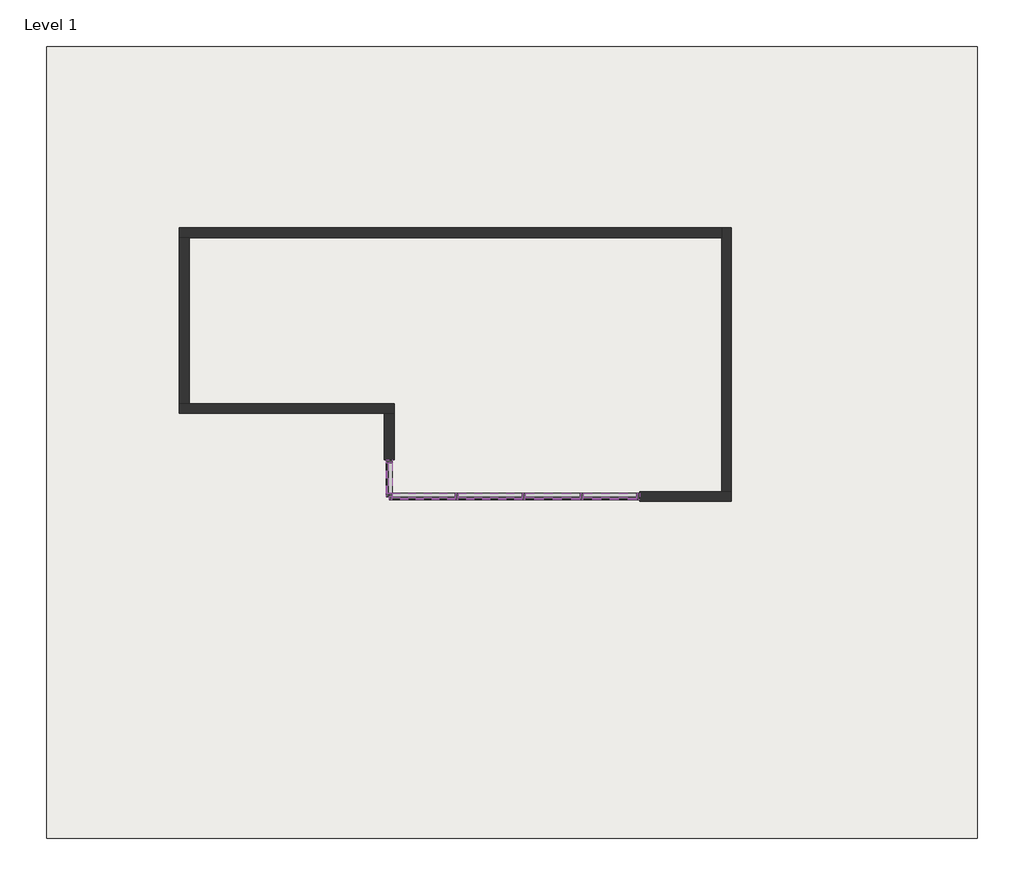
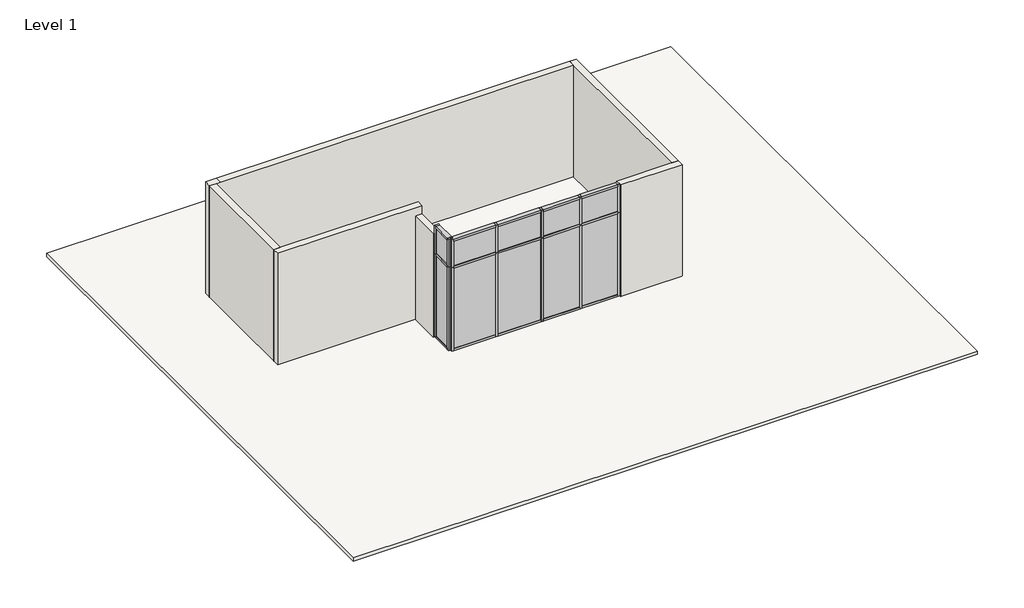
# One storey: 29 members, 10 plates, 6 walls, 1 slab.
"""IFC4 building model written with IfcOpenShell, lengths in millimetres."""

from ifc_helpers import new_model, si_unit, frame, origin, origin_with_axes, place, context, project, spatial, polyline, outline, extrude, faceted_brep, transform, mapped, element, save
from components import member_afc9459e, member_f32bdbca, member_44103a32, member_65750824, member_73c23c35, member_5e365d0c, member_923d5781, member_a78380a5, member_12300432, member_410c6227, member_d6aa3d2f, member_6609bf83, member_48e25eb9, member_c84aaad6, system_panel_glazed_120799d7, system_panel_glazed_8e2f599f, system_panel_glazed_26227597, system_panel_glazed_1d091053, system_panel_glazed_c9ee7fb0, system_panel_glazed_e21b380e, system_panel_glazed_be7f0fdb, system_panel_glazed_03477ef2, system_panel_glazed_aebd10dd, system_panel_glazed_a205a7ab

model = new_model("IFC4")

# Units and contexts
model_context = context("Model", 3, world=origin())
ifc_project = project(units=[si_unit("LENGTHUNIT", "METRE", prefix="MILLI")], contexts=[model_context])

# Site, building, storey
site = spatial("IfcSite", under=ifc_project)
building = spatial("IfcBuilding", under=site)
storey = spatial("IfcBuildingStorey", under=building, Name="Level 1", Elevation=0.0)

# Members
placement = place(None, origin())
member_shape = member_afc9459e(model_context)
element("IfcMember", 1, ObjectType="Rectangular Mullion : 2.5\" x 5\" rectangular", at=placement, inside=storey, context=model_context, shape_type="MappedRepresentation", body=[
    mapped(member_shape, transform((-8475.461895, 635.561619, 2743.2), x_axis=(0.0, 0.0, 1.0), y_axis=(0.0, 1.0, 0.0), z_axis=(-1.0, 0.0, 0.0))),
])
member_2_shape = member_f32bdbca(model_context)
element("IfcMember", 2, ObjectType="Rectangular Mullion : 2.5\" x 5\" rectangular", at=placement, inside=storey, context=model_context, shape_type="MappedRepresentation", body=[
    mapped(member_2_shape, transform((-8475.461895, 635.561619, 3657.6), x_axis=(0.0, 0.0, 1.0), y_axis=(0.0, 1.0, 0.0), z_axis=(-1.0, 0.0, 0.0))),
])
member_3_shape = member_44103a32(model_context)
element("IfcMember", 3, ObjectType="Rectangular Mullion : 2.5\" x 5\" rectangular", at=placement, inside=storey, context=model_context, shape_type="MappedRepresentation", body=[
    mapped(member_3_shape, transform((-9840.711895, 635.561619, 2743.2), x_axis=(0.0, 0.0, 1.0), y_axis=(0.0, 1.0, 0.0), z_axis=(-1.0, 0.0, 0.0))),
])
member_4_shape = member_65750824(model_context)
element("IfcMember", 4, ObjectType="Rectangular Mullion : 2.5\" x 5\" rectangular", at=placement, inside=storey, context=model_context, shape_type="MappedRepresentation", body=[
    mapped(member_4_shape, transform((-9840.711895, 635.561619, 3657.6), x_axis=(0.0, 0.0, 1.0), y_axis=(0.0, 1.0, 0.0), z_axis=(-1.0, 0.0, 0.0))),
])
member_5_shape = member_73c23c35(model_context)
element("IfcMember", 5, ObjectType="Rectangular Mullion : 2.5\" x 5\" rectangular", at=placement, inside=storey, context=model_context, shape_type="MappedRepresentation", body=[
    mapped(member_5_shape, transform((-9904.211895, 635.561619, 2743.2), x_axis=(-1.0, 0.0, 0.0), y_axis=(0.0, 1.0, 0.0), z_axis=(0.0, 0.0, -1.0))),
])
element("IfcMember", 6, ObjectType="Rectangular Mullion : 2.5\" x 5\" rectangular", at=placement, inside=storey, context=model_context, shape_type="MappedRepresentation", body=[
    mapped(member_5_shape, transform((-9904.211895, 1397.561619, 2743.2), x_axis=(0.0, 1.0, 0.0), y_axis=(1.0, 0.0, 0.0), z_axis=(0.0, 0.0, -1.0))),
])
member_6_shape = member_5e365d0c(model_context)
element("IfcMember", 7, ObjectType="Rectangular Mullion : 2.5\" x 5\" rectangular", at=placement, inside=storey, context=model_context, shape_type="MappedRepresentation", body=[
    mapped(member_6_shape, transform((-9904.211895, 1334.061619, 3657.6), x_axis=(0.0, 0.0, 1.0), y_axis=(1.0, 0.0, 0.0), z_axis=(0.0, 1.0, 0.0))),
])
element("IfcMember", 8, ObjectType="Rectangular Mullion : 2.5\" x 5\" rectangular", at=placement, inside=storey, context=model_context, shape_type="MappedRepresentation", body=[
    mapped(member_5_shape, transform((-9904.211895, 635.561619, 3657.6), x_axis=(0.0, -1.0, 0.0), y_axis=(1.0, 0.0, 0.0), z_axis=(0.0, 0.0, 1.0))),
])
element("IfcMember", 9, ObjectType="Rectangular Mullion : 2.5\" x 5\" rectangular", at=placement, inside=storey, context=model_context, shape_type="MappedRepresentation", body=[
    mapped(member_5_shape, transform((-4698.461546, 635.561619, 3657.6), x_axis=(1.0, 0.0, 0.0), y_axis=(0.0, 1.0, 0.0), z_axis=(0.0, 0.0, 1.0))),
])
member_7_shape = member_923d5781(model_context)
element("IfcMember", 10, ObjectType="Rectangular Mullion : 2.5\" x 5\" rectangular", at=placement, inside=storey, context=model_context, shape_type="MappedRepresentation", body=[
    mapped(member_7_shape, transform((-8507.211895, 635.561619, 0.0), x_axis=(-1.0, 0.0, 0.0), y_axis=(0.0, 1.0, 0.0), z_axis=(0.0, 0.0, -1.0))),
])
element("IfcMember", 11, ObjectType="Rectangular Mullion : 2.5\" x 5\" rectangular", at=placement, inside=storey, context=model_context, shape_type="MappedRepresentation", body=[
    mapped(member_7_shape, transform((-7110.211895, 635.561619, 0.0), x_axis=(-1.0, 0.0, 0.0), y_axis=(0.0, 1.0, 0.0), z_axis=(0.0, 0.0, -1.0))),
])
element("IfcMember", 12, ObjectType="Rectangular Mullion : 2.5\" x 5\" rectangular", at=placement, inside=storey, context=model_context, shape_type="MappedRepresentation", body=[
    mapped(member_7_shape, transform((-5904.3367205, 635.561619, 0.0), x_axis=(-1.0, 0.0, 0.0), y_axis=(0.0, 1.0, 0.0), z_axis=(0.0, 0.0, -1.0))),
])
element("IfcMember", 13, ObjectType="Rectangular Mullion : 2.5\" x 5\" rectangular", at=placement, inside=storey, context=model_context, shape_type="MappedRepresentation", body=[
    mapped(member_4_shape, transform((-8538.961895, 635.561619, 0.0), x_axis=(0.0, 0.0, -1.0), y_axis=(0.0, 1.0, 0.0), z_axis=(1.0, 0.0, 0.0))),
])
element("IfcMember", 14, ObjectType="Rectangular Mullion : 2.5\" x 5\" rectangular", at=placement, inside=storey, context=model_context, shape_type="MappedRepresentation", body=[
    mapped(member_2_shape, transform((-7141.961895, 635.561619, 0.0), x_axis=(0.0, 0.0, -1.0), y_axis=(0.0, 1.0, 0.0), z_axis=(1.0, 0.0, 0.0))),
])
member_8_shape = member_a78380a5(model_context)
element("IfcMember", 15, ObjectType="Rectangular Mullion : 2.5\" x 5\" rectangular", at=placement, inside=storey, context=model_context, shape_type="MappedRepresentation", body=[
    mapped(member_8_shape, transform((-9904.211895, 635.561619, 0.0), x_axis=(-1.0, 0.0, 0.0), y_axis=(0.0, 1.0, 0.0), z_axis=(0.0, 0.0, -1.0))),
])
element("IfcMember", 16, ObjectType="Rectangular Mullion : 2.5\" x 5\" rectangular", at=placement, inside=storey, context=model_context, shape_type="MappedRepresentation", body=[
    mapped(member_8_shape, transform((-9904.211895, 1397.561619, 0.0), x_axis=(0.0, 1.0, 0.0), y_axis=(1.0, 0.0, 0.0), z_axis=(0.0, 0.0, -1.0))),
])
element("IfcMember", 17, ObjectType="Rectangular Mullion : 2.5\" x 5\" rectangular", at=placement, inside=storey, context=model_context, shape_type="MappedRepresentation", body=[
    mapped(member_8_shape, transform((-4698.461546, 635.561619, 2743.2), x_axis=(1.0, 0.0, 0.0), y_axis=(0.0, 1.0, 0.0), z_axis=(0.0, 0.0, 1.0))),
])
element("IfcMember", 18, ObjectType="Rectangular Mullion : 2.5\" x 5\" rectangular", at=placement, inside=storey, context=model_context, shape_type="MappedRepresentation", body=[
    mapped(member_8_shape, transform((-9904.211895, 635.561619, 2743.2), x_axis=(0.0, -1.0, 0.0), y_axis=(1.0, 0.0, 0.0), z_axis=(0.0, 0.0, 1.0))),
])
element("IfcMember", 19, ObjectType="Rectangular Mullion : 2.5\" x 5\" rectangular", at=placement, inside=storey, context=model_context, shape_type="MappedRepresentation", body=[
    mapped(member_6_shape, transform((-9904.211895, 699.061619, 0.0), x_axis=(0.0, 0.0, -1.0), y_axis=(1.0, 0.0, 0.0), z_axis=(0.0, -1.0, 0.0))),
])
member_9_shape = member_12300432(model_context)
element("IfcMember", 20, ObjectType="Rectangular Mullion : 2.5\" x 5\" rectangular", at=placement, inside=storey, context=model_context, shape_type="MappedRepresentation", body=[
    mapped(member_9_shape, transform((-9904.211895, 1334.061619, 2743.2), x_axis=(0.0, 0.0, 1.0), y_axis=(1.0, 0.0, 0.0), z_axis=(0.0, 1.0, 0.0))),
])
member_10_shape = member_410c6227(model_context)
element("IfcMember", 21, ObjectType="Rectangular Mullion : 2.5\" x 5\" rectangular", at=placement, inside=storey, context=model_context, shape_type="MappedRepresentation", body=[
    mapped(member_10_shape, transform((-8507.211895, 635.561619, 2743.2), x_axis=(-1.0, 0.0, 0.0), y_axis=(0.0, 1.0, 0.0), z_axis=(0.0, 0.0, -1.0))),
])
element("IfcMember", 22, ObjectType="Rectangular Mullion : 2.5\" x 5\" rectangular", at=placement, inside=storey, context=model_context, shape_type="MappedRepresentation", body=[
    mapped(member_10_shape, transform((-7110.211895, 635.561619, 2743.2), x_axis=(-1.0, 0.0, 0.0), y_axis=(0.0, 1.0, 0.0), z_axis=(0.0, 0.0, -1.0))),
])
element("IfcMember", 23, ObjectType="Rectangular Mullion : 2.5\" x 5\" rectangular", at=placement, inside=storey, context=model_context, shape_type="MappedRepresentation", body=[
    mapped(member_10_shape, transform((-5904.3367205, 635.561619, 2743.2), x_axis=(-1.0, 0.0, 0.0), y_axis=(0.0, 1.0, 0.0), z_axis=(0.0, 0.0, -1.0))),
])
member_11_shape = member_d6aa3d2f(model_context)
element("IfcMember", 24, ObjectType="Rectangular Mullion : 2.5\" x 5\" rectangular", at=placement, inside=storey, context=model_context, shape_type="MappedRepresentation", body=[
    mapped(member_11_shape, transform((-5872.5867205, 635.561619, 2743.2), x_axis=(0.0, 0.0, 1.0), y_axis=(0.0, 1.0, 0.0), z_axis=(-1.0, 0.0, 0.0))),
])
member_12_shape = member_6609bf83(model_context)
element("IfcMember", 25, ObjectType="Rectangular Mullion : 2.5\" x 5\" rectangular", at=placement, inside=storey, context=model_context, shape_type="MappedRepresentation", body=[
    mapped(member_12_shape, transform((-7078.461895, 635.561619, 3657.6), x_axis=(0.0, 0.0, 1.0), y_axis=(0.0, 1.0, 0.0), z_axis=(-1.0, 0.0, 0.0))),
])
member_13_shape = member_48e25eb9(model_context)
element("IfcMember", 26, ObjectType="Rectangular Mullion : 2.5\" x 5\" rectangular", at=placement, inside=storey, context=model_context, shape_type="MappedRepresentation", body=[
    mapped(member_13_shape, transform((-4761.961546, 635.561619, 0.0), x_axis=(0.0, 0.0, -1.0), y_axis=(0.0, 1.0, 0.0), z_axis=(1.0, 0.0, 0.0))),
])
member_14_shape = member_c84aaad6(model_context)
element("IfcMember", 27, ObjectType="Rectangular Mullion : 2.5\" x 5\" rectangular", at=placement, inside=storey, context=model_context, shape_type="MappedRepresentation", body=[
    mapped(member_14_shape, transform((-7078.461895, 635.561619, 2743.2), x_axis=(0.0, 0.0, 1.0), y_axis=(0.0, 1.0, 0.0), z_axis=(-1.0, 0.0, 0.0))),
])
element("IfcMember", 28, ObjectType="Rectangular Mullion : 2.5\" x 5\" rectangular", at=placement, inside=storey, context=model_context, shape_type="MappedRepresentation", body=[
    mapped(member_13_shape, transform((-5872.5867205, 635.561619, 3657.6), x_axis=(0.0, 0.0, 1.0), y_axis=(0.0, 1.0, 0.0), z_axis=(-1.0, 0.0, 0.0))),
])
element("IfcMember", 29, ObjectType="Rectangular Mullion : 2.5\" x 5\" rectangular", at=placement, inside=storey, context=model_context, shape_type="MappedRepresentation", body=[
    mapped(member_12_shape, transform((-5936.0867205, 635.561619, 0.0), x_axis=(0.0, 0.0, -1.0), y_axis=(0.0, 1.0, 0.0), z_axis=(1.0, 0.0, 0.0))),
])

# Plates
system_panel_glazed_shape = system_panel_glazed_120799d7(model_context)
element("IfcPlate", 30, ObjectType="System Panel : Glazed", at=placement, inside=storey, context=model_context, shape_type="MappedRepresentation", body=[
    mapped(system_panel_glazed_shape, transform((-9189.836895, 635.561619, 63.5), x_axis=(-1.0, 0.0, 0.0), y_axis=(0.0, -1.0, 0.0), z_axis=(0.0, 0.0, 1.0))),
])
system_panel_glazed_2_shape = system_panel_glazed_8e2f599f(model_context)
element("IfcPlate", 31, ObjectType="System Panel : Glazed", at=placement, inside=storey, context=model_context, shape_type="MappedRepresentation", body=[
    mapped(system_panel_glazed_2_shape, transform((-7808.711895, 635.561619, 63.5), x_axis=(-1.0, 0.0, 0.0), y_axis=(0.0, -1.0, 0.0), z_axis=(0.0, 0.0, 1.0))),
])
system_panel_glazed_3_shape = system_panel_glazed_26227597(model_context)
element("IfcPlate", 32, ObjectType="System Panel : Glazed", at=placement, inside=storey, context=model_context, shape_type="MappedRepresentation", body=[
    mapped(system_panel_glazed_3_shape, transform((-9904.211895, 1016.561619, 63.5), x_axis=(0.0, 1.0, 0.0), y_axis=(-1.0, 0.0, 0.0), z_axis=(0.0, 0.0, 1.0))),
])
system_panel_glazed_4_shape = system_panel_glazed_1d091053(model_context)
element("IfcPlate", 33, ObjectType="System Panel : Glazed", at=placement, inside=storey, context=model_context, shape_type="MappedRepresentation", body=[
    mapped(system_panel_glazed_4_shape, transform((-9904.211895, 1016.561619, 2774.95), x_axis=(0.0, 1.0, 0.0), y_axis=(-1.0, 0.0, 0.0), z_axis=(0.0, 0.0, 1.0))),
])
system_panel_glazed_5_shape = system_panel_glazed_c9ee7fb0(model_context)
element("IfcPlate", 34, ObjectType="System Panel : Glazed", at=placement, inside=storey, context=model_context, shape_type="MappedRepresentation", body=[
    mapped(system_panel_glazed_5_shape, transform((-9189.836895, 635.561619, 2774.95), x_axis=(-1.0, 0.0, 0.0), y_axis=(0.0, -1.0, 0.0), z_axis=(0.0, 0.0, 1.0))),
])
system_panel_glazed_6_shape = system_panel_glazed_e21b380e(model_context)
element("IfcPlate", 35, ObjectType="System Panel : Glazed", at=placement, inside=storey, context=model_context, shape_type="MappedRepresentation", body=[
    mapped(system_panel_glazed_6_shape, transform((-7808.711895, 635.561619, 2774.95), x_axis=(-1.0, 0.0, 0.0), y_axis=(0.0, -1.0, 0.0), z_axis=(0.0, 0.0, 1.0))),
])
system_panel_glazed_7_shape = system_panel_glazed_be7f0fdb(model_context)
element("IfcPlate", 36, ObjectType="System Panel : Glazed", at=placement, inside=storey, context=model_context, shape_type="MappedRepresentation", body=[
    mapped(system_panel_glazed_7_shape, transform((-6507.2743078, 635.561619, 63.5), x_axis=(-1.0, 0.0, 0.0), y_axis=(0.0, -1.0, 0.0), z_axis=(0.0, 0.0, 1.0))),
])
system_panel_glazed_8_shape = system_panel_glazed_03477ef2(model_context)
element("IfcPlate", 37, ObjectType="System Panel : Glazed", at=placement, inside=storey, context=model_context, shape_type="MappedRepresentation", body=[
    mapped(system_panel_glazed_8_shape, transform((-6507.2743078, 635.561619, 2774.95), x_axis=(-1.0, 0.0, 0.0), y_axis=(0.0, -1.0, 0.0), z_axis=(0.0, 0.0, 1.0))),
])
system_panel_glazed_9_shape = system_panel_glazed_aebd10dd(model_context)
element("IfcPlate", 38, ObjectType="System Panel : Glazed", at=placement, inside=storey, context=model_context, shape_type="MappedRepresentation", body=[
    mapped(system_panel_glazed_9_shape, transform((-5317.2741332, 635.561619, 63.5), x_axis=(-1.0, 0.0, 0.0), y_axis=(0.0, -1.0, 0.0), z_axis=(0.0, 0.0, 1.0))),
])
system_panel_glazed_10_shape = system_panel_glazed_a205a7ab(model_context)
element("IfcPlate", 39, ObjectType="System Panel : Glazed", at=placement, inside=storey, context=model_context, shape_type="MappedRepresentation", body=[
    mapped(system_panel_glazed_10_shape, transform((-5317.2741332, 635.561619, 2774.95), x_axis=(-1.0, 0.0, 0.0), y_axis=(0.0, -1.0, 0.0), z_axis=(0.0, 0.0, 1.0))),
])

# Slab
element("IfcSlab", 40, ObjectType="LW Concrete on Metal Deck", at=placement, inside=storey, context=model_context, shape_type="SweptSolid", body=[
    extrude(outline(polyline([(2322.9035909, 9991.2265954), (2322.9035909, -6467.9734046), (-17031.8964091, -6467.9734046), (-17031.8964091, 9991.2265954), (2322.9035909, 9991.2265954)])), frame((0.0, 0.0, -104.775), z_axis=(0.0, 0.0, 1.0), x_axis=(1.0, 0.0, 0.0)), (0.0, 0.0, 1.0), 104.775),
])

# Walls
element("IfcWall", 41, ObjectType="Generic - 8\"", at=placement, inside=storey, context=model_context, shape_type="Brep", body=[
    faceted_brep([(-14273.011895, 6020.361619, 0.0), (-14069.811895, 6020.361619, 0.0), (-2995.411895, 6020.361619, 0.0), (-2995.411895, 6020.361619, 3657.6), (-13942.811895, 6020.361619, 3657.6), (-14069.811895, 6020.361619, 3657.6), (-14273.011895, 6020.361619, 3657.6), (-14273.011895, 6223.561619, 0.0), (-14273.011895, 6223.561619, 3657.6), (-13942.811895, 6223.561619, 3657.6), (-2995.411895, 6223.561619, 3657.6), (-2995.411895, 6223.561619, 0.0)], [[[0, 1, 2, 3, 4, 5, 6]], [[7, 8, 9, 10, 11]], [[2, 1, 0, 7, 11]], [[0, 6, 8, 7]], [[3, 2, 11, 10]], [[6, 5, 4, 9, 8]], [[4, 3, 10, 9]]]),
])
element("IfcWall", 42, ObjectType="Generic - 8\"", at=placement, inside=storey, context=model_context, shape_type="SweptSolid", body=[
    extrude(outline(polyline([(-14069.811895, 6020.361619), (-14069.811895, 2565.961619), (-14273.011895, 2565.961619), (-14273.011895, 6020.361619), (-14069.811895, 6020.361619)])), origin_with_axes(), (0.0, 0.0, 1.0), 3657.6),
])
element("IfcWall", 43, ObjectType="Generic - 8\"", at=placement, inside=storey, context=model_context, shape_type="Brep", body=[
    faceted_brep([(-2792.211895, 737.161619, 0.0), (-2995.411895, 737.161619, 0.0), (-4698.461546, 737.161619, 0.0), (-4698.461546, 737.161619, 3657.6), (-2995.411895, 737.161619, 3657.6), (-2792.211895, 737.161619, 3657.6), (-2792.211895, 533.961619, 0.0), (-2792.211895, 533.961619, 3657.6), (-4698.461546, 533.961619, 3657.6), (-4698.461546, 533.961619, 0.0)], [[[0, 1, 2, 3, 4, 5]], [[6, 7, 8, 9]], [[0, 5, 7, 6]], [[5, 4, 3, 8, 7]], [[2, 1, 0, 6, 9]], [[3, 2, 9, 8]]]),
])
element("IfcWall", 44, ObjectType="Generic - 8\"", at=placement, inside=storey, context=model_context, shape_type="Brep", body=[
    faceted_brep([(-2995.411895, 6223.561619, 0.0), (-2995.411895, 6020.361619, 0.0), (-2995.411895, 737.161619, 0.0), (-2995.411895, 737.161619, 3657.6), (-2995.411895, 6020.361619, 3657.6), (-2995.411895, 6223.561619, 3657.6), (-2792.211895, 6223.561619, 0.0), (-2792.211895, 6223.561619, 3657.6), (-2792.211895, 737.161619, 3657.6), (-2792.211895, 737.161619, 0.0)], [[[0, 1, 2, 3, 4, 5]], [[6, 7, 8, 9]], [[2, 1, 0, 6, 9]], [[0, 5, 7, 6]], [[3, 2, 9, 8]], [[5, 4, 3, 8, 7]]]),
])
element("IfcWall", 45, ObjectType="Generic - 8\"", at=placement, inside=storey, context=model_context, shape_type="Brep", body=[
    faceted_brep([(-14273.011895, 2362.761619, 0.0), (-10005.811895, 2362.761619, 0.0), (-9802.611895, 2362.761619, 0.0), (-9802.611895, 2362.761619, 3390.8435953), (-9802.611895, 2362.761619, 3657.6), (-14273.011895, 2362.761619, 3657.6), (-14273.011895, 2565.961619, 0.0), (-14273.011895, 2565.961619, 3657.6), (-14069.811895, 2565.961619, 3657.6), (-9802.611895, 2565.961619, 3657.6), (-9802.611895, 2565.961619, 0.0), (-14069.811895, 2565.961619, 0.0)], [[[0, 1, 2, 3, 4, 5]], [[6, 7, 8, 9, 10, 11]], [[2, 1, 0, 6, 11, 10]], [[5, 4, 9, 8, 7]], [[0, 5, 7, 6]], [[4, 3, 2, 10, 9]]]),
])
element("IfcWall", 46, ObjectType="Generic - 8\"", at=placement, inside=storey, context=model_context, shape_type="SweptSolid", body=[
    extrude(outline(polyline([(-10005.811895, 1397.561619), (-10005.811895, 2362.761619), (-9802.611895, 2362.761619), (-9802.611895, 1397.561619), (-10005.811895, 1397.561619)])), origin_with_axes(), (0.0, 0.0, 1.0), 3390.8435953),
])

save(model, "model.ifc")

# Revit data of these elements
# Type "Rectangular Mullion : 2.5\" x 5\" rectangular"
#   built-in parameter 1007304 = 0.416667 (stored number, unit not read)
#   built-in parameter 1007301 = 0.104167 (stored number, unit not read)
#   built-in parameter 1007300 = 0.104167 (stored number, unit not read)
# Type "System Panel : Glazed"
#   Construction Type Id = "GSP4R"
#   Analytic Construction = "1/8 in Pilkington single glazing"
#   Visual Light Transmittance = 0.9
#   Solar Heat Gain Coefficient = 0.86
#   Heat Transfer Coefficient (U) = 1.18115 BTU/(h·ft²·°F)
# Type "LW Concrete on Metal Deck"
#   Assembly Code = "B1010"
#   Function = 0
#   Layers, outside or top first: 0' - 4" "Concrete, Lightweight" (function 1); 0' - 0 1/8" "Metal Deck" (function 1)
# Type "Generic - 8\""
#   Assembly Code = "B2010"
#   Layers, outside or top first: 0' - 8" no material (function 1)
# Elements 1, 2, 3, 4, 5, 6, 7, 8, 9, 10, 11, 12, 13, 14, 15, 16, 17, 18, 19, 20, 21, 22, 23, 24, 25, 26, 27, 28, 29 (IfcMember, "Rectangular Mullion : 2.5\" x 5\" rectangular")
#   Phase Created = New Construction
#   Materials on its faces: "Aluminum"
# Elements 30, 31, 32, 33, 34, 35, 36, 37, 38, 39 (IfcPlate, "System Panel : Glazed")
#   Phase Created = New Construction
#   Materials on its faces: "Glass"
# Element 40 (IfcSlab, "LW Concrete on Metal Deck")
#   Height Offset From Level = 0' - 0"
#   Phase Created = New Construction
#   Materials on its faces: "Metal Deck", "Concrete, Lightweight"
# Elements 41, 42, 44, 45 (IfcWall, "Generic - 8\"")
#   Top Offset = 0' - 0"
#   Base Offset = 0' - 0"
#   Unconnected Height = 12' - 0"
#   wall height = 12' - 0"
#   Phase Created = New Construction
#   Base Constraint = Level 1
#   Materials on its faces: "Default Wall", "Cherry"
# Element 43 (IfcWall, "Generic - 8\"")
#   Top Offset = 0' - 0"
#   Base Offset = 0' - 0"
#   Unconnected Height = 12' - 0"
#   wall height = 12' - 0"
#   Phase Created = New Construction
#   Base Constraint = Level 1
#   Materials on its faces: "Default Wall", "Cherry", "Gypsum Wall Board"
# Element 46 (IfcWall, "Generic - 8\"")
#   Top Offset = 0' - 0"
#   Base Offset = 0' - 0"
#   Unconnected Height = 11' - 1.49778"
#   wall height = 11' - 1.49778"
#   Phase Created = New Construction
#   Base Constraint = Level 1
#   Materials on its faces: "Default Wall", "Cherry"
# Materials
#   "Concrete, Lightweight": class "Concrete", colour RGB 142 141 140, transparency 0, Description = "Lightweight concrete", Cost = 0
#   "Metal Deck": class "Metal", colour RGB 199 199 199, transparency 0, Description = "Steel, mill finish", Cost = 0
#   "Aluminum": class "Metal", colour RGB 247 247 247, transparency 0, Description = "Aluminum 6061", Cost = 0
#   "Glass": class "Glass", colour RGB 0 128 192, transparency 0.75, Description = "Soda Lime Glass", Cost = 0
#   "Default Wall": colour RGB 128 128 128, transparency 0
#   "Cherry": class "Wood", colour RGB 226 177 128, transparency 0, Description = "Prunus Serotina", Cost = 0
#   "Gypsum Wall Board": class "Generic", colour RGB 127 127 127, transparency 0, Description = "Gypsum Wall Board", Cost = 0
